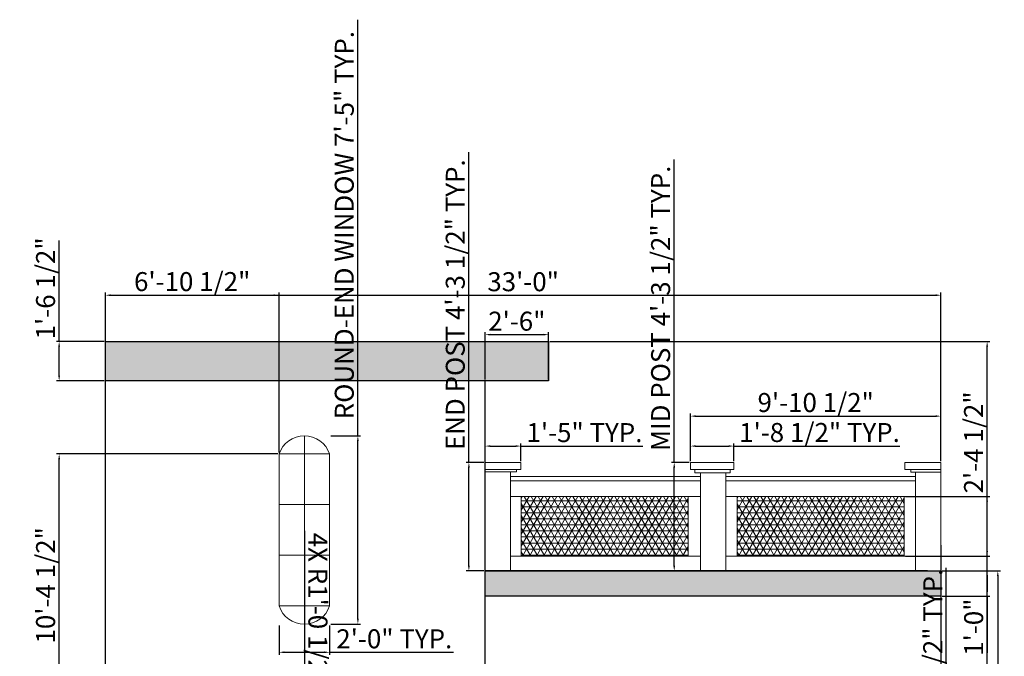
# Model space of a CAD drawing. Units: inches. Extents: x 107 to 1375, y 131 to 922.
# Tile 4 of 4: x 821 to 1287, y 621 to 922. Entities that reach past the tile are written whole.
import ezdxf

# ---------------------------------------------------------------- set-up
doc = ezdxf.new("R2010")
doc.units = ezdxf.units.IN
for name, color, linetype, lineweight in [('A-ANNO-DIMS', 2, 'Continuous', 13), ('A-ELEV', 7, 'Continuous', 30), ('A-ELEV-RAIL', 7, 'Continuous', 18), ('A-GLAZ-ELEV', 4, 'Continuous', 18), ('A-ROOF-ELEV', 7, 'Continuous', 30)]:
    doc.layers.add(name, color=color, linetype=linetype, lineweight=lineweight)
doc.layers.add('A-ELEV-PATT', color=18, linetype='Continuous', lineweight=13, true_color=0x000000)
doc.styles.get("Standard").update_dxf_attribs({"font": 'arial.ttf'})
doc.dimstyles.new('ISO-25', dxfattribs={"dimtxt": 9, "dimasz": 2.5, "dimexe": 1.25, "dimexo": 0.625, "dimtad": 1, "dimlunit": 3, "dimtxsty": 'Standard', "dimcen": 2.5, "dimadec": 0, "dimazin": 0, "dimtfac": 1, "dimtmove": 0, "dimatfit": 3, "dimfxl": 1, "dimarcsym": 0})

# ---------------------------------------------------------------- blocks, each defined once
blk = doc.blocks.new('*D6')
at = {"layer": 'A-ANNO-DIMS', "color": 0, "lineweight": -2, "transparency": 16777216}
for p, q in [((1257.76, 661.18), (1285.35, 661.18)), ((1284.1, 658.68), (1284.1, 393.68)), ((1257.76, 391.18), (1285.35, 391.18))]:
    blk.add_line(p, q, dxfattribs=at)
at = {"layer": 'A-ANNO-DIMS', "color": 0, "transparency": 16777216}
for points in [[(1283.69, 658.68), (1284.52, 658.68), (1284.1, 661.18)], [(1283.69, 393.68), (1284.52, 393.68), (1284.1, 391.18)]]:
    blk.add_solid(points, dxfattribs=at)
at = {"layer": 'Defpoints', "color": 0, "transparency": 16777216}
for p in [(1257.14, 661.18), (1257.14, 391.18), (1284.1, 391.18)]:
    blk.add_point(p, dxfattribs=at)
at = {"layer": 'A-ANNO-DIMS', "color": 0, "transparency": 16777216, "insert": (1278.88, 526.18), "char_height": 9, "attachment_point": 5, "rotation": 90}
blk.add_mtext('22\'-6"', dxfattribs=at)
blk = doc.blocks.new('WINDOW-ELEV-ROUND-END')
for p, q in [((12, 89.15), (12, 0)), ((0, 80.57), (0, 8.57)), ((24, 80.57), (0, 80.57)), ((24, 8.57), (24, 80.57)), ((24, 56.57), (0, 56.57)), ((24, 32.57), (0, 32.57)), ((24, 8.57), (0, 8.57))]:
    blk.add_line(p, q)
for centre, start, end in [((12, 76.46), 18.9145, 161.0855), ((12, 12.68), 198.9145, 341.0855)]:
    blk.add_arc(centre, 12.68, start, end)
blk = doc.blocks.new('GUARD-POST-LEFT')
for p, q in [((16.93, 51.4), (0, 51.4)), ((0, 51.4), (0, 48)), ((16.93, 48), (16.93, 51.4)), ((0, 48), (0, 0)), ((0, 48), (16.93, 48)), ((0, 46.97), (14.82, 46.97)), ((12, 46.97), (12, 0)), ((14.82, 46.97), (14.82, 48))]:
    blk.add_line(p, q)
blk = doc.blocks.new('GUARD-POST-CENTER')
for p, q in [((0, 51.4), (20.53, 51.4)), ((0, 51.4), (0, 48)), ((20.53, 48), (20.53, 51.4)), ((0, 48), (20.53, 48)), ((1.99, 48), (1.99, 46.37)), ((18.83, 46.37), (18.83, 48)), ((1.99, 46.37), (18.83, 46.37)), ((4.69, 0), (4.69, 46.37)), ((16.69, 0), (16.69, 46.37))]:
    blk.add_line(p, q)
blk = doc.blocks.new('GUARD-CAP-RIGHT')
for p, q in [((17.1, 4.57), (0, 4.57)), ((0, 4.57), (0, 1.16)), ((17.1, 1.16), (0, 1.16)), ((2.86, 1.16), (2.86, 0)), ((2.86, 0), (17.1, 0)), ((17.1, 1.16), (17.1, 4.57))]:
    blk.add_line(p, q)
blk = doc.blocks.new('*D36')
at = {"layer": 'A-ANNO-DIMS', "color": 0, "lineweight": -2, "transparency": 16777216}
for p, q in [((980.81, 725.14), (980.81, 922.27)), ((968.07, 725.14), (982.06, 725.14)), ((980.81, 638.5), (980.81, 722.64)), ((968.07, 636), (982.06, 636))]:
    blk.add_line(p, q, dxfattribs=at)
at = {"layer": 'A-ANNO-DIMS', "color": 0, "transparency": 16777216}
for points in [[(980.4, 722.64), (981.23, 722.64), (980.81, 725.14)], [(980.4, 638.5), (981.23, 638.5), (980.81, 636)]]:
    blk.add_solid(points, dxfattribs=at)
at = {"layer": 'Defpoints', "color": 0, "transparency": 16777216}
for p in [(967.44, 725.14), (980.81, 725.14), (967.44, 636)]:
    blk.add_point(p, dxfattribs=at)
at = {"layer": 'A-ANNO-DIMS', "color": 0, "transparency": 16777216, "insert": (975.53, 824.96), "char_height": 9, "attachment_point": 5, "rotation": 90}
blk.add_mtext('ROUND-END WINDOW 7\'-5" TYP.', dxfattribs=at)
blk = doc.blocks.new('*D37')
at = {"layer": 'A-ANNO-DIMS', "color": 0, "lineweight": -2, "transparency": 16777216}
for p, q in [((943.44, 635.37), (943.44, 621.37)), ((967.44, 635.37), (967.44, 621.37)), ((945.94, 622.62), (964.94, 622.62)), ((967.44, 622.62), (1026.2, 622.62))]:
    blk.add_line(p, q, dxfattribs=at)
at = {"layer": 'A-ANNO-DIMS', "color": 0, "transparency": 16777216}
for points in [[(945.94, 623.04), (945.94, 622.21), (943.44, 622.62)], [(964.94, 623.04), (964.94, 622.21), (967.44, 622.62)]]:
    blk.add_solid(points, dxfattribs=at)
at = {"layer": 'Defpoints', "color": 0, "transparency": 16777216}
for p in [(943.44, 636), (967.44, 636), (967.44, 622.62)]:
    blk.add_point(p, dxfattribs=at)
at = {"layer": 'A-ANNO-DIMS', "color": 0, "transparency": 16777216, "insert": (998.07, 627.84), "char_height": 9, "attachment_point": 5}
blk.add_mtext('2\'-0" TYP.', dxfattribs=at)
blk = doc.blocks.new('*D40')
at = {"layer": 'A-ANNO-DIMS', "color": 0, "lineweight": -2, "transparency": 16777216}
for p, q in [((1033.43, 712.58), (1033.43, 859.46)), ((1040.51, 712.58), (1032.18, 712.58)), ((1033.43, 663.68), (1033.43, 710.08)), ((1040.51, 661.18), (1032.18, 661.18))]:
    blk.add_line(p, q, dxfattribs=at)
at = {"layer": 'A-ANNO-DIMS', "color": 0, "transparency": 16777216}
for points in [[(1033.01, 710.08), (1033.84, 710.08), (1033.43, 712.58)], [(1033.01, 663.68), (1033.84, 663.68), (1033.43, 661.18)]]:
    blk.add_solid(points, dxfattribs=at)
at = {"layer": 'Defpoints', "color": 0, "transparency": 16777216}
for p in [(1033.43, 712.58), (1041.14, 712.58), (1041.14, 661.18)]:
    blk.add_point(p, dxfattribs=at)
at = {"layer": 'A-ANNO-DIMS', "color": 0, "transparency": 16777216, "insert": (1028.14, 787.27), "char_height": 9, "attachment_point": 5, "rotation": 90}
blk.add_mtext('END POST 4\'-3 1/2" TYP.', dxfattribs=at)
blk = doc.blocks.new('*D41')
at = {"layer": 'A-ANNO-DIMS', "color": 0, "lineweight": -2, "transparency": 16777216}
for p, q in [((1041.14, 713.21), (1041.14, 721.54)), ((1043.64, 720.29), (1055.57, 720.29)), ((1058.07, 713.21), (1058.07, 721.54)), ((1058.07, 720.29), (1115.83, 720.29))]:
    blk.add_line(p, q, dxfattribs=at)
at = {"layer": 'A-ANNO-DIMS', "color": 0, "transparency": 16777216}
for points in [[(1043.64, 720.71), (1043.64, 719.88), (1041.14, 720.29)], [(1055.57, 720.71), (1055.57, 719.88), (1058.07, 720.29)]]:
    blk.add_solid(points, dxfattribs=at)
at = {"layer": 'Defpoints', "color": 0, "transparency": 16777216}
for p in [(1058.07, 720.29), (1041.14, 712.58), (1058.07, 712.58)]:
    blk.add_point(p, dxfattribs=at)
at = {"layer": 'A-ANNO-DIMS', "color": 0, "transparency": 16777216, "insert": (1088.2, 725.51), "char_height": 9, "attachment_point": 5}
blk.add_mtext('1\'-5" TYP.', dxfattribs=at)
blk = doc.blocks.new('*D42')
at = {"layer": 'A-ANNO-DIMS', "color": 0, "lineweight": -2, "transparency": 16777216}
for p, q in [((1130.74, 712.58), (1130.74, 856.02)), ((1137.83, 712.58), (1129.49, 712.58)), ((1130.74, 663.68), (1130.74, 710.08)), ((1137.83, 661.18), (1129.49, 661.18))]:
    blk.add_line(p, q, dxfattribs=at)
at = {"layer": 'A-ANNO-DIMS', "color": 0, "transparency": 16777216}
for points in [[(1130.32, 710.08), (1131.16, 710.08), (1130.74, 712.58)], [(1130.32, 663.68), (1131.16, 663.68), (1130.74, 661.18)]]:
    blk.add_solid(points, dxfattribs=at)
at = {"layer": 'Defpoints', "color": 0, "transparency": 16777216}
for p in [(1130.74, 712.58), (1138.45, 712.58), (1138.45, 661.18)]:
    blk.add_point(p, dxfattribs=at)
at = {"layer": 'A-ANNO-DIMS', "color": 0, "transparency": 16777216, "insert": (1125.46, 785.55), "char_height": 9, "attachment_point": 5, "rotation": 90}
blk.add_mtext('MID POST 4\'-3 1/2" TYP.', dxfattribs=at)
blk = doc.blocks.new('*D43')
at = {"layer": 'A-ANNO-DIMS', "color": 0, "lineweight": -2, "transparency": 16777216}
for p, q in [((1138.45, 713.21), (1138.45, 721.54)), ((1140.95, 720.29), (1156.48, 720.29)), ((1158.98, 713.21), (1158.98, 721.54)), ((1158.98, 720.29), (1237.71, 720.29))]:
    blk.add_line(p, q, dxfattribs=at)
at = {"layer": 'A-ANNO-DIMS', "color": 0, "transparency": 16777216}
for points in [[(1140.95, 720.71), (1140.95, 719.88), (1138.45, 720.29)], [(1156.48, 720.71), (1156.48, 719.88), (1158.98, 720.29)]]:
    blk.add_solid(points, dxfattribs=at)
at = {"layer": 'Defpoints', "color": 0, "transparency": 16777216}
for p in [(1158.98, 720.29), (1138.45, 712.58), (1158.98, 712.58)]:
    blk.add_point(p, dxfattribs=at)
at = {"layer": 'A-ANNO-DIMS', "color": 0, "transparency": 16777216, "insert": (1199.6, 725.57), "char_height": 9, "attachment_point": 5}
blk.add_mtext('1\'-8 1/2" TYP.', dxfattribs=at)
blk = doc.blocks.new('*D45')
at = {"layer": 'A-ANNO-DIMS', "color": 0, "lineweight": -2, "transparency": 16777216}
for p, q in [((1259.7, 583.08), (1259.7, 662.66)), ((1257.76, 580.58), (1260.95, 580.58)), ((1259.7, 576.02), (1259.7, 580.58)), ((1257.76, 576.02), (1260.95, 576.02)), ((1259.7, 573.52), (1259.7, 571.02))]:
    blk.add_line(p, q, dxfattribs=at)
at = {"layer": 'A-ANNO-DIMS', "color": 0, "transparency": 16777216}
for points in [[(1259.28, 583.08), (1260.12, 583.08), (1259.7, 580.58)], [(1259.28, 573.52), (1260.12, 573.52), (1259.7, 576.02)]]:
    blk.add_solid(points, dxfattribs=at)
at = {"layer": 'Defpoints', "color": 0, "transparency": 16777216}
for p in [(1257.14, 580.58), (1259.7, 580.58), (1257.14, 576.02)]:
    blk.add_point(p, dxfattribs=at)
at = {"layer": 'A-ANNO-DIMS', "color": 0, "transparency": 16777216, "insert": (1254.42, 624.12), "char_height": 9, "attachment_point": 5, "rotation": 90}
blk.add_mtext('0\'-4 1/2" TYP.', dxfattribs=at)
blk = doc.blocks.new('*D57')
at = {"layer": 'A-ANNO-DIMS', "color": 0, "lineweight": -2, "transparency": 16777216}
for p, q in [((861.14, 770.49), (861.14, 793.01)), ((863.64, 791.76), (1254.64, 791.76)), ((1257.14, 713.21), (1257.14, 793.01))]:
    blk.add_line(p, q, dxfattribs=at)
at = {"layer": 'A-ANNO-DIMS', "color": 0, "transparency": 16777216}
for points in [[(863.64, 792.18), (863.64, 791.35), (861.14, 791.76)], [(1254.64, 792.18), (1254.64, 791.35), (1257.14, 791.76)]]:
    blk.add_solid(points, dxfattribs=at)
at = {"layer": 'Defpoints', "color": 0, "transparency": 16777216}
for p in [(1257.14, 791.76), (861.14, 769.86), (1257.14, 712.58)]:
    blk.add_point(p, dxfattribs=at)
at = {"layer": 'A-ANNO-DIMS', "color": 0, "transparency": 16777216, "insert": (1059.14, 796.99), "char_height": 9, "attachment_point": 5}
blk.add_mtext('33\'-0"', dxfattribs=at)
blk = doc.blocks.new('*D58')
at = {"layer": 'A-ANNO-DIMS', "color": 0, "lineweight": -2, "transparency": 16777216}
for p, q in [((1071.8, 769.86), (1280.29, 769.86)), ((1279.04, 352.56), (1279.04, 767.36)), ((1257.76, 350.06), (1280.29, 350.06))]:
    blk.add_line(p, q, dxfattribs=at)
at = {"layer": 'A-ANNO-DIMS', "color": 0, "transparency": 16777216}
for points in [[(1278.62, 767.36), (1279.45, 767.36), (1279.04, 769.86)], [(1278.62, 352.56), (1279.45, 352.56), (1279.04, 350.06)]]:
    blk.add_solid(points, dxfattribs=at)
at = {"layer": 'Defpoints', "color": 0, "transparency": 16777216}
for p in [(1071.17, 769.86), (1279.04, 769.86), (1257.14, 350.06)]:
    blk.add_point(p, dxfattribs=at)
at = {"layer": 'A-ANNO-DIMS', "color": 0, "transparency": 16777216, "insert": (1273.81, 559.96), "char_height": 9, "attachment_point": 5, "rotation": 90}
blk.add_mtext('35\'-0"', dxfattribs=at)
blk = doc.blocks.new('*D66')
at = {"layer": 'A-ANNO-DIMS', "color": 0, "lineweight": -2, "transparency": 16777216}
for p, q in [((942.82, 716.57), (837.99, 716.57)), ((839.24, 594.62), (839.24, 714.07)), ((942.82, 592.12), (837.99, 592.12))]:
    blk.add_line(p, q, dxfattribs=at)
at = {"layer": 'A-ANNO-DIMS', "color": 0, "transparency": 16777216}
for points in [[(838.82, 714.07), (839.65, 714.07), (839.24, 716.57)], [(838.82, 594.62), (839.65, 594.62), (839.24, 592.12)]]:
    blk.add_solid(points, dxfattribs=at)
at = {"layer": 'Defpoints', "color": 0, "transparency": 16777216}
for p in [(839.24, 716.57), (943.44, 716.57), (943.44, 592.12)]:
    blk.add_point(p, dxfattribs=at)
at = {"layer": 'A-ANNO-DIMS', "color": 0, "transparency": 16777216, "insert": (833.96, 654.34), "char_height": 9, "attachment_point": 5, "rotation": 90}
blk.add_mtext('10\'-4 1/2"', dxfattribs=at)
blk = doc.blocks.new('*D69')
at = {"layer": 'A-ANNO-DIMS', "color": 0, "lineweight": -2, "transparency": 16777216}
for p, q in [((861.14, 751.8), (861.14, 793.01)), ((863.64, 791.76), (940.94, 791.76)), ((943.44, 717.19), (943.44, 793.01))]:
    blk.add_line(p, q, dxfattribs=at)
at = {"layer": 'A-ANNO-DIMS', "color": 0, "transparency": 16777216}
for points in [[(863.64, 792.18), (863.64, 791.35), (861.14, 791.76)], [(940.94, 792.18), (940.94, 791.35), (943.44, 791.76)]]:
    blk.add_solid(points, dxfattribs=at)
at = {"layer": 'Defpoints', "color": 0, "transparency": 16777216}
for p in [(943.44, 791.76), (861.14, 751.18), (943.44, 716.57)]:
    blk.add_point(p, dxfattribs=at)
at = {"layer": 'A-ANNO-DIMS', "color": 0, "transparency": 16777216, "insert": (902.29, 797.04), "char_height": 9, "attachment_point": 5}
blk.add_mtext('6\'-10 1/2"', dxfattribs=at)
blk = doc.blocks.new('*D70')
at = {"layer": 'A-ANNO-DIMS', "color": 0, "lineweight": -2, "transparency": 16777216}
for p, q in [((1138.45, 713.21), (1138.45, 735.73)), ((1140.95, 734.48), (1254.64, 734.48)), ((1257.14, 713.21), (1257.14, 735.73))]:
    blk.add_line(p, q, dxfattribs=at)
at = {"layer": 'A-ANNO-DIMS', "color": 0, "transparency": 16777216}
for points in [[(1140.95, 734.9), (1140.95, 734.07), (1138.45, 734.48)], [(1254.64, 734.9), (1254.64, 734.07), (1257.14, 734.48)]]:
    blk.add_solid(points, dxfattribs=at)
at = {"layer": 'Defpoints', "color": 0, "transparency": 16777216}
for p in [(1257.14, 734.48), (1138.45, 712.58), (1257.14, 712.58)]:
    blk.add_point(p, dxfattribs=at)
at = {"layer": 'A-ANNO-DIMS', "color": 0, "transparency": 16777216, "insert": (1197.79, 739.76), "char_height": 9, "attachment_point": 5}
blk.add_mtext('9\'-10 1/2"', dxfattribs=at)
blk = doc.blocks.new('*D71')
at = {"layer": 'A-ANNO-DIMS', "color": 0, "lineweight": -2, "transparency": 16777216}
for p, q in [((1041.14, 751.8), (1041.14, 774.33)), ((1043.64, 773.08), (1068.67, 773.08)), ((1071.17, 751.8), (1071.17, 774.33))]:
    blk.add_line(p, q, dxfattribs=at)
at = {"layer": 'A-ANNO-DIMS', "color": 0, "transparency": 16777216}
for points in [[(1043.64, 773.5), (1043.64, 772.66), (1041.14, 773.08)], [(1068.67, 773.5), (1068.67, 772.66), (1071.17, 773.08)]]:
    blk.add_solid(points, dxfattribs=at)
at = {"layer": 'Defpoints', "color": 0, "transparency": 16777216}
for p in [(1071.17, 773.08), (1041.14, 751.18), (1071.17, 751.18)]:
    blk.add_point(p, dxfattribs=at)
at = {"layer": 'A-ANNO-DIMS', "color": 0, "transparency": 16777216, "insert": (1056.15, 778.3), "char_height": 9, "attachment_point": 5}
blk.add_mtext('2\'-6"', dxfattribs=at)
blk = doc.blocks.new('*D74')
at = {"layer": 'A-ANNO-DIMS', "color": 0, "lineweight": -2, "transparency": 16777216}
for p, q in [((1279.04, 696.4), (1279.04, 745.2)), ((1240.42, 696.4), (1280.29, 696.4)), ((1279.04, 670.61), (1279.04, 693.9)), ((1240.42, 668.11), (1280.29, 668.11))]:
    blk.add_line(p, q, dxfattribs=at)
at = {"layer": 'A-ANNO-DIMS', "color": 0, "transparency": 16777216}
for points in [[(1278.62, 693.9), (1279.45, 693.9), (1279.04, 696.4)], [(1278.62, 670.61), (1279.45, 670.61), (1279.04, 668.11)]]:
    blk.add_solid(points, dxfattribs=at)
at = {"layer": 'Defpoints', "color": 0, "transparency": 16777216}
for p in [(1239.8, 696.4), (1279.04, 696.4), (1239.8, 668.11)]:
    blk.add_point(p, dxfattribs=at)
at = {"layer": 'A-ANNO-DIMS', "color": 0, "transparency": 16777216, "insert": (1273.76, 722.05), "char_height": 9, "attachment_point": 5, "rotation": 90}
blk.add_mtext('2\'-4 1/2"', dxfattribs=at)
blk = doc.blocks.new('*D75')
at = {"layer": 'A-ANNO-DIMS', "color": 0, "lineweight": -2, "transparency": 16777216}
for p, q in [((839.24, 769.86), (839.24, 817.66)), ((860.51, 769.86), (837.99, 769.86)), ((839.24, 753.68), (839.24, 767.36)), ((860.51, 751.18), (837.99, 751.18))]:
    blk.add_line(p, q, dxfattribs=at)
at = {"layer": 'A-ANNO-DIMS', "color": 0, "transparency": 16777216}
for points in [[(838.82, 767.36), (839.65, 767.36), (839.24, 769.86)], [(838.82, 753.68), (839.65, 753.68), (839.24, 751.18)]]:
    blk.add_solid(points, dxfattribs=at)
at = {"layer": 'Defpoints', "color": 0, "transparency": 16777216}
for p in [(839.24, 769.86), (861.14, 769.86), (861.14, 751.18)]:
    blk.add_point(p, dxfattribs=at)
at = {"layer": 'A-ANNO-DIMS', "color": 0, "transparency": 16777216, "insert": (833.96, 795.01), "char_height": 9, "attachment_point": 5, "rotation": 90}
blk.add_mtext('1\'-6 1/2"', dxfattribs=at)
blk = doc.blocks.new('*D76')
at = {"layer": 'A-ANNO-DIMS', "color": 0, "lineweight": -2, "transparency": 16777216}
for p, q in [((1257.76, 661.18), (1280.29, 661.18)), ((1279.04, 658.68), (1279.04, 651.68)), ((1257.76, 649.18), (1280.29, 649.18)), ((1279.04, 649.18), (1279.04, 622.35))]:
    blk.add_line(p, q, dxfattribs=at)
at = {"layer": 'A-ANNO-DIMS', "color": 0, "transparency": 16777216}
for points in [[(1278.62, 658.68), (1279.45, 658.68), (1279.04, 661.18)], [(1278.62, 651.68), (1279.45, 651.68), (1279.04, 649.18)]]:
    blk.add_solid(points, dxfattribs=at)
at = {"layer": 'Defpoints', "color": 0, "transparency": 16777216}
for p in [(1257.14, 661.18), (1257.14, 649.18), (1279.04, 649.18)]:
    blk.add_point(p, dxfattribs=at)
at = {"layer": 'A-ANNO-DIMS', "color": 0, "transparency": 16777216, "insert": (1273.82, 634.52), "char_height": 9, "attachment_point": 5, "rotation": 90}
blk.add_mtext('1\'-0"', dxfattribs=at)
blk = doc.blocks.new('*D81')
at = {"layer": 'A-ANNO-DIMS', "color": 0, "lineweight": -2, "transparency": 16777216}
for p, q in [((955.44, 680.15), (955.44, 603.19)), ((955.44, 588.01), (955.44, 600.69))]:
    blk.add_line(p, q, dxfattribs=at)
at = {"layer": 'A-ANNO-DIMS', "color": 0, "transparency": 16777216}
blk.add_solid([(955.86, 603.19), (955.02, 603.19), (955.44, 600.69)], dxfattribs=at)
at = {"layer": 'Defpoints', "color": 0, "transparency": 16777216}
for p in [(955.44, 600.69), (955.44, 588.01)]:
    blk.add_point(p, dxfattribs=at)
at = {"layer": 'A-ANNO-DIMS', "color": 0, "transparency": 16777216, "insert": (960.72, 642.92), "char_height": 9, "attachment_point": 5, "rotation": 270.0018}
blk.add_mtext('4X R1\'-0 1/2"', dxfattribs=at)

msp = doc.modelspace()

# ---------------------------------------------------------------- hatches: boundary and pattern name
at = {"layer": 'A-ELEV-PATT'}
h = msp.add_hatch(color=256, dxfattribs=at)
h.dxf.hatch_style = 1
h.paths.add_polyline_path([(1071.173, 769.862), (861.136, 769.862), (861.136, 751.179), (1041.136, 751.179), (1071.173, 751.179)])
h = msp.add_hatch(dxfattribs=at)
h.set_pattern_fill('NET3', color=256, scale=0.9)
h.paths.add_polyline_path([(1137.409, 696.403), (1058.258, 696.403), (1058.258, 668.106), (1137.409, 668.106)])
h.paths.add_polyline_path([(1239.797, 696.403), (1160.646, 696.403), (1160.646, 668.106), (1239.797, 668.106)])
h = msp.add_hatch(color=256, dxfattribs=at)
h.dxf.hatch_style = 1
h.paths.add_polyline_path([(1257.136, 661.179), (1041.136, 661.179), (1041.136, 649.179), (1257.136, 649.179)])
h.paths.add_polyline_path([(1257.136, 529.179), (1041.136, 529.179), (1041.136, 517.179), (1257.136, 517.179)])

# ---------------------------------------------------------------- linework, layer by layer
at = {"layer": 'A-ELEV'}
for p, q in [((861.136, 391.179), (861.136, 751.179)), ((1041.136, 391.179), (1041.136, 751.179)), ((1257.136, 673.43), (1257.136, 394.43)), ((1250.832, 661.179), (1041.136, 661.179)), ((1041.136, 661.179), (1257.136, 661.179)), ((1257.136, 649.179), (1041.136, 649.179))]:
    msp.add_line(p, q, dxfattribs=at)
at = {"layer": 'A-ELEV-RAIL'}
for p, q in [((1053.136, 705.817), (1143.136, 705.817)), ((1155.136, 705.817), (1245.136, 705.817)), ((1245.136, 661.179), (1245.136, 708.015)), ((1257.136, 661.179), (1257.136, 709.179)), ((1053.136, 703.817), (1143.136, 703.817)), ((1155.136, 703.817), (1245.136, 703.817)), ((1053.136, 696.403), (1058.258, 696.403)), ((1137.409, 696.403), (1143.136, 696.403)), ((1160.646, 696.403), (1155.136, 696.403)), ((1239.797, 696.403), (1245.136, 696.403)), ((1058.258, 668.106), (1053.136, 668.106)), ((1137.409, 668.106), (1143.136, 668.106)), ((1160.646, 668.106), (1155.136, 668.106)), ((1239.797, 668.106), (1245.136, 668.106))]:
    msp.add_line(p, q, dxfattribs=at)
for points in [[(1058.258, 696.403), (1137.409, 696.403), (1137.409, 668.106), (1058.258, 668.106)], [(1160.646, 696.403), (1239.797, 696.403), (1239.797, 668.106), (1160.646, 668.106)]]:
    msp.add_lwpolyline(points, close=True, dxfattribs=at)
at = {"layer": 'A-ROOF-ELEV'}
for p, q in [((861.136, 751.179), (861.136, 769.862)), ((861.136, 769.862), (1071.173, 769.862)), ((1071.173, 769.862), (1071.173, 751.179)), ((1041.136, 751.179), (861.136, 751.179)), ((1071.173, 751.179), (1041.136, 751.179))]:
    msp.add_line(p, q, dxfattribs=at)

# ---------------------------------------------------------------- block references
at = {"layer": 'A-ELEV-RAIL'}
for name, p in [('GUARD-POST-LEFT', (1041.136, 661.179)), ('GUARD-POST-CENTER', (1138.451, 661.179)), ('GUARD-CAP-RIGHT', (1240.04, 708.015))]:
    msp.add_blockref(name, p, dxfattribs=at)
at = {"layer": 'A-GLAZ-ELEV'}
msp.add_blockref('WINDOW-ELEV-ROUND-END', (943.44, 635.997), dxfattribs=at)

# ---------------------------------------------------------------- dimensions: what is measured, and where the dimension line sits
at = {"layer": 'A-ANNO-DIMS'}
for base, p1, p2, text, picture, middle in [((980.812, 725.143), (967.44, 635.997), (967.44, 725.143), 'ROUND-END WINDOW <> TYP.', '*D36', (975.531, 824.956)), ((1033.425, 712.583), (1041.136, 661.179), (1041.136, 712.583), 'END POST <> TYP.', '*D40', (1028.141, 787.269)), ((1130.74, 712.583), (1138.451, 661.179), (1138.451, 712.583), 'MID POST <> TYP.', '*D42', (1125.456, 785.55)), ((1259.701, 580.583), (1257.136, 576.015), (1257.136, 580.583), '<> TYP.', '*D45', (1254.422, 624.123))]:
    dim = msp.add_linear_dim(base=base, p1=p1, p2=p2, angle=90, text=text, dimstyle='ISO-25', override={"dimdec": 1, "dimlfac": 1, "dimrnd": 0, "dimzin": 1, "dimdsep": 46, "dimlunit": 4, "dimfrac": 2}, dxfattribs=at)
    dim.commit()
    dim.dimension.update_dxf_attribs({"geometry": picture, "text_midpoint": middle})
for base, p1, p2, angle, override, picture, middle in [((839.236, 769.862), (861.136, 751.179), (861.136, 769.862), 90, {"dimdec": 1, "dimlfac": 1, "dimrnd": 0, "dimzin": 1, "dimdsep": 46, "dimlunit": 4, "dimfrac": 2}, '*D75', (833.958, 795.011)), ((1071.173, 773.079), (1041.136, 751.179), (1071.173, 751.179), 0, {"dimdec": 1, "dimlfac": 1, "dimrnd": 0, "dimzin": 1, "dimdsep": 46, "dimlunit": 4, "dimfrac": 2}, '*D71', (1056.154, 778.299)), ((1279.036, 769.862), (1257.136, 350.065), (1071.173, 769.862), 90, {"dimdec": 1, "dimlfac": 1, "dimrnd": 0, "dimzin": 1, "dimdsep": 46, "dimlunit": 4, "dimfrac": 2}, '*D58', (1273.813, 559.963)), ((1257.136, 734.483), (1138.451, 712.583), (1257.136, 712.583), 0, {"dimdec": 1, "dimlfac": 1, "dimrnd": 0, "dimzin": 1, "dimdsep": 46, "dimlunit": 4, "dimfrac": 2}, '*D70', (1197.793, 739.762)), ((1279.036, 696.403), (1239.797, 668.106), (1239.797, 696.403), 90, {"dimdec": 1, "dimlfac": 1, "dimrnd": 0, "dimzin": 1, "dimdsep": 46, "dimlunit": 4, "dimfrac": 2}, '*D74', (1273.758, 722.053)), ((839.236, 716.57), (943.44, 592.118), (943.44, 716.57), 90, {"dimdec": 1, "dimlfac": 1, "dimrnd": 0, "dimzin": 1, "dimdsep": 46, "dimlunit": 4, "dimfrac": 2}, '*D66', (833.958, 654.344)), ((1284.102, 391.179), (1257.136, 661.179), (1257.136, 391.179), 90, {"dimclrd": 0, "dimclre": 0, "dimclrt": 0}, '*D6', (1278.882, 526.179)), ((1279.036, 649.179), (1257.136, 661.179), (1257.136, 649.179), 90, {"dimdec": 1, "dimlfac": 1, "dimrnd": 0, "dimzin": 1, "dimdsep": 46, "dimlunit": 4, "dimfrac": 2}, '*D76', (1273.816, 634.516))]:
    dim = msp.add_linear_dim(base=base, p1=p1, p2=p2, angle=angle, dimstyle='ISO-25', override=override, dxfattribs=at)
    dim.commit()
    dim.dimension.update_dxf_attribs({"geometry": picture, "text_midpoint": middle})
for base, p1, p2, picture, middle in [((943.44, 791.762), (861.136, 751.179), (943.44, 716.57), '*D69', (902.288, 797.041)), ((1257.136, 791.762), (861.136, 769.862), (1257.136, 712.583), '*D57', (1059.136, 796.985))]:
    dim = msp.add_linear_dim(base=base, p1=p1, p2=p2, dimstyle='ISO-25', override={"dimdec": 1, "dimlfac": 1, "dimrnd": 0, "dimzin": 1, "dimdsep": 46, "dimlunit": 4, "dimfrac": 2}, dxfattribs=at)
    dim.commit()
    dim.dimension.update_dxf_attribs({"geometry": picture, "text_midpoint": middle})
for base, p1, p2, picture, middle in [((1158.98, 720.294), (1138.451, 712.583), (1158.98, 712.583), '*D43', (1199.597, 725.572)), ((1058.067, 720.294), (1041.136, 712.583), (1058.067, 712.583), '*D41', (1088.199, 725.514)), ((967.44, 622.625), (943.44, 635.997), (967.44, 635.997), '*D37', (998.072, 627.845))]:
    dim = msp.add_linear_dim(base=base, p1=p1, p2=p2, text='<> TYP.', dimstyle='ISO-25', override={"dimdec": 1, "dimlfac": 1, "dimrnd": 0, "dimzin": 1, "dimdsep": 46, "dimlunit": 4, "dimfrac": 2}, dxfattribs=at)
    dim.commit()
    dim.dimension.update_dxf_attribs({"geometry": picture, "text_midpoint": middle})
dim = msp.add_radius_dim(center=(955.44, 588.006), mpoint=(955.44, 600.691), text='4X <>', dimstyle='ISO-25', override={"dimdec": 1, "dimlfac": 1, "dimrnd": 0, "dimzin": 1, "dimdsep": 46, "dimlunit": 4, "dimfrac": 2}, dxfattribs=at)
dim.commit()
dim.dimension.update_dxf_attribs({"geometry": '*D81', "text_midpoint": (960.717, 642.92)})

doc.saveas('drawing.dxf')
